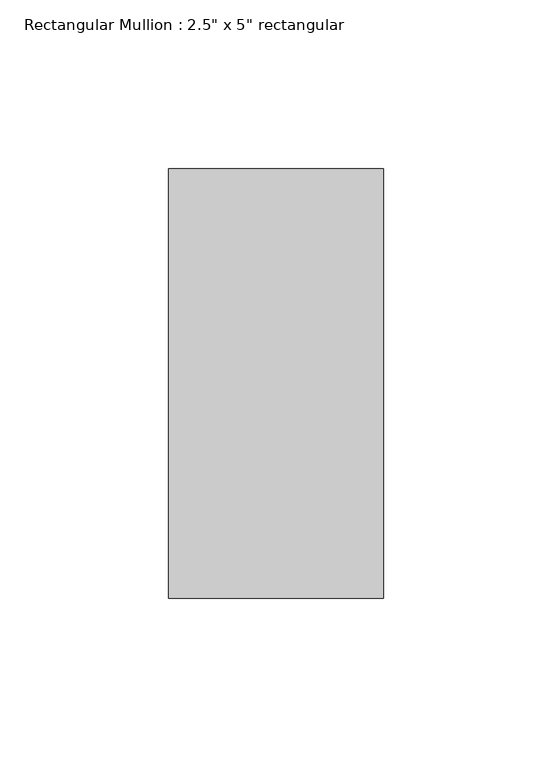
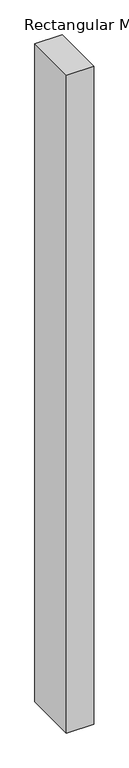
"""IFC4 building model written with IfcOpenShell, lengths in millimetres: member geometry."""

from ifc_helpers import new_model, si_unit, frame, origin, place, context, project, spatial, polyline, outline, extrude, source, transform, mapped, element, save


def member_94b81e23(model_context):
    return source(origin(), model_context, "Body", "SweptSolid", [
        extrude(outline(polyline([(31.75, 63.5), (31.75, -63.5), (-31.75, -63.5), (-31.75, 63.5), (31.75, 63.5)])), frame((0.0, 0.0, -1620.8138027), z_axis=(0.0, 0.0, 1.0), x_axis=(1.0, 0.0, 0.0)), (0.0, 0.0, 1.0), 1620.8138027),
    ])


if __name__ == "__main__":
    model = new_model("IFC4")
    model_context = context("Model", 3, world=origin())
    ifc_project = project(units=[si_unit("LENGTHUNIT", "METRE", prefix="MILLI")], contexts=[model_context])
    site = spatial("IfcSite", under=ifc_project)
    building = spatial("IfcBuilding", under=site)
    placement = place(None, origin())
    member_shape = member_94b81e23(model_context)
    element("IfcMember", 1, ObjectType="Rectangular Mullion : 2.5\" x 5\" rectangular", at=placement, inside=building, context=model_context, shape_type="MappedRepresentation", body=[
        mapped(member_shape, transform((0.0, 0.0, 0.0), x_axis=(1.0, 0.0, 0.0), y_axis=(0.0, 1.0, 0.0), z_axis=(0.0, 0.0, 1.0))),
    ])
    save(model, "model.ifc")

# Revit data of these elements
# Type "Rectangular Mullion : 2.5\" x 5\" rectangular"
#   built-in parameter 1007304 = 0.416667 (stored number, unit not read)
#   built-in parameter 1007301 = 0.104167 (stored number, unit not read)
#   built-in parameter 1007300 = 0.104167 (stored number, unit not read)
# Element 1 (IfcMember, "Rectangular Mullion : 2.5\" x 5\" rectangular")
#   Materials on its faces: "Aluminum"
# Materials
#   "Aluminum": class "Metal", colour RGB 247 247 247, transparency 0, Description = "Aluminum 6061", Cost = 0
